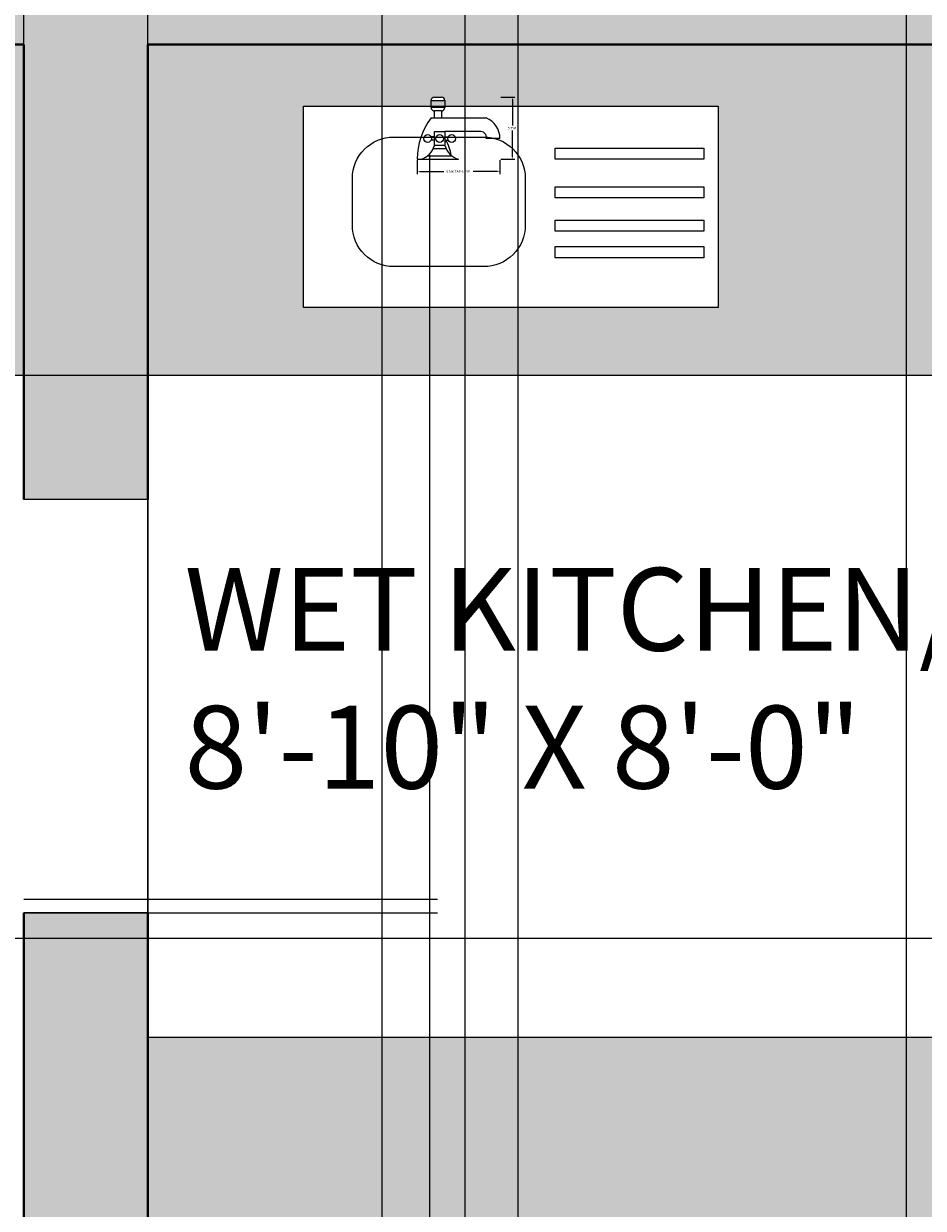
# Model space of a CAD drawing. Units: inches. Extents: x 818 to 1898, y 976 to 2364.
# Tile 89 of 96: x 1591 to 1656, y 1960 to 2046. Entities that reach past the tile are written whole.
import ezdxf

# ---------------------------------------------------------------- set-up
doc = ezdxf.new("R2010")
doc.units = ezdxf.units.IN
doc.header["$LTSCALE"] = 5
doc.header["$MEASUREMENT"] = 0
for name, color, linetype, lineweight in [('A-ANNO-DIMS', 2, 'Continuous', 18), ('A-AREA-IDEN', 7, 'Continuous', 18), ('A-DOOR', 3, 'Continuous', 25), ('A-FLOR-CASE', 8, 'Continuous', 18), ('A-FLOR-FIXT', 9, 'Continuous', 18), ('A-FURN-PATT', 8, 'Continuous', 9), ('A-WALL', 7, 'Continuous', 40)]:
    doc.layers.add(name, color=color, linetype=linetype, lineweight=lineweight)
doc.layers.add('A-WALL-PATT', color=251, linetype='Continuous', lineweight=13, true_color=0x636466)
doc.styles.get("Standard").update_dxf_attribs({"font": 'arial.ttf'})
doc.dimstyles.get("Standard").update_dxf_attribs({"dimtxt": 0.18, "dimasz": 0.18, "dimexe": 0.18, "dimexo": 0.0625, "dimgap": 0.09, "dimtad": 0, "dimtih": 1, "dimtoh": 1, "dimdec": 4, "dimzin": 0, "dimdsep": 46, "dimtxsty": 'Standard', "dimcen": 0.09, "dimadec": 0, "dimazin": 0, "dimtfac": 1, "dimtdec": 4, "dimtofl": 0, "dimtmove": 0, "dimatfit": 3, "dimfxl": 1, "dimtolj": 1, "dimtzin": 0, "dimarcsym": 0})

# ---------------------------------------------------------------- blocks, each defined once
blk = doc.blocks.new('Faucet - Bathroom side')
for p, q in [((-0.625, 4.25), (0.375, 4.25)), ((0.375, 3.75), (-0.625, 3.75)), ((-0.375, 3), (-0.375, 3.5)), ((0.125, 3.5), (0.125, 3)), ((-0.625, 3), (3.375, 3)), ((2.875, 2), (0.375, 2)), ((-0.375, 1.625), (-0.625, 1.625)), ((-0.375, 1.375), (-0.625, 1.375)), ((0.375, 1.625), (0.625, 1.625)), ((0.375, 1.375), (0.625, 1.375)), ((4.375, 1.5), (3.375, 1.5)), ((-1.625, 0), (-1.375, 0)), ((-1.375, 0), (1.375, 0)), ((-0.88366, 0.25), (0.88424, 0.25)), ((0.48078, 0.75), (-0.47286, 0.75))]:
    blk.add_line(p, q)
for points in [[(-0.375, 4.5), (0.125, 4.5)], [(-0.625, 3.75), (-0.625, 4.25)], [(0.125, 3.5), (-0.375, 3.5)], [(0.375, 4.25), (0.375, 3.75)]]:
    blk.add_lwpolyline(points)
blk.add_lwpolyline([(-0.375, 1), (-0.375, 2), (0.375, 2), (0.375, 1)], close=True)
for centre in [(-0.875, 1.5), (0, 1.5), (0.875, 1.5)]:
    blk.add_circle(centre, 0.27951)
for centre, radius, start, end in [((-0.38253, 4.2575), 0.24259, 88.22243, 181.7776), ((0.13252, 4.2575), 0.24259, 358.2224, 91.77757), ((-0.38253, 3.7424), 0.24259, 178.2224, 271.7776), ((0.13252, 3.7424), 0.24259, 268.2224, 1.777565), ((3.45929, -0.0281), 5.08436, 143.4467, 179.6834), ((2.70708, 1.4714), 1.66816, 0.9827695, 66.39737), ((2.96867, 1.5936), 0.41699, 347.0192, 102.9808), ((-1.75, 1.375), 1.42522, 285.2551, 344.7449), ((1.75, 1.375), 1.42522, 195.2551, 254.7449), ((-2.49562, -0.286), 3.38273, 9.709485, 29.48735)]:
    blk.add_arc(centre, radius, start, end)
blk = doc.blocks.new('*D38')
at = {"layer": 'A-ANNO-DIMS', "color": 0, "lineweight": -2, "ltscale": 5, "transparency": 16777216}
for p, q in [((1619.259, 2035.688), (1619.259, 2034.671)), ((1625.259, 2035.688), (1625.259, 2034.671)), ((1619.439, 2034.851), (1621.193, 2034.851)), ((1625.079, 2034.851), (1623.324, 2034.851))]:
    blk.add_line(p, q, dxfattribs=at)
at = {"layer": 'A-ANNO-DIMS', "color": 0, "ltscale": 5, "transparency": 16777216}
for points in [[(1619.439, 2034.881), (1619.439, 2034.821), (1619.259, 2034.851)], [(1625.079, 2034.881), (1625.079, 2034.821), (1625.259, 2034.851)]]:
    blk.add_solid(points, dxfattribs=at)
at = {"layer": 'Defpoints', "color": 0, "ltscale": 5, "transparency": 16777216}
for p in [(1619.259, 2035.751), (1625.259, 2035.751), (1625.259, 2034.851)]:
    blk.add_point(p, dxfattribs=at)
at = {"layer": 'A-ANNO-DIMS', "color": 0, "ltscale": 5, "transparency": 16777216, "insert": (1622.259, 2034.851), "char_height": 0.18, "attachment_point": 5}
blk.add_mtext('\\A1;SINK TAP 6 TYP.', dxfattribs=at)
blk = doc.blocks.new('*D39')
at = {"layer": 'A-ANNO-DIMS', "color": 0, "lineweight": -2, "ltscale": 5, "transparency": 16777216}
for p, q in [((1625.321, 2040.253), (1626.339, 2040.253)), ((1626.159, 2040.073), (1626.159, 2038.184)), ((1626.159, 2035.931), (1626.159, 2037.82)), ((1625.321, 2035.751), (1626.339, 2035.751))]:
    blk.add_line(p, q, dxfattribs=at)
at = {"layer": 'A-ANNO-DIMS', "color": 0, "ltscale": 5, "transparency": 16777216}
for points in [[(1626.129, 2040.073), (1626.189, 2040.073), (1626.159, 2040.253)], [(1626.129, 2035.931), (1626.189, 2035.931), (1626.159, 2035.751)]]:
    blk.add_solid(points, dxfattribs=at)
at = {"layer": 'Defpoints', "color": 0, "ltscale": 5, "transparency": 16777216}
for p in [(1625.259, 2040.253), (1626.159, 2040.253), (1625.259, 2035.751)]:
    blk.add_point(p, dxfattribs=at)
at = {"layer": 'A-ANNO-DIMS', "color": 0, "ltscale": 5, "transparency": 16777216, "insert": (1626.159, 2038.002), "char_height": 0.18, "attachment_point": 5}
blk.add_mtext('\\A1;5 TYP.', dxfattribs=at)
blk = doc.blocks.new('*D85')
at = {"layer": 'A-ANNO-DIMS', "color": 0, "lineweight": -2, "ltscale": 5, "transparency": 16777216}
for p, q in [((1258.788, 2053.078), (1897.916, 2053.078)), ((1897.736, 2052.898), (1897.736, 1876.76)), ((1897.736, 1700.258), (1897.736, 1876.396)), ((1258.788, 1700.078), (1897.916, 1700.078))]:
    blk.add_line(p, q, dxfattribs=at)
at = {"layer": 'A-ANNO-DIMS', "color": 0, "ltscale": 5, "transparency": 16777216}
for points in [[(1897.706, 2052.898), (1897.766, 2052.898), (1897.736, 2053.078)], [(1897.706, 1700.258), (1897.766, 1700.258), (1897.736, 1700.078)]]:
    blk.add_solid(points, dxfattribs=at)
at = {"layer": 'Defpoints', "color": 0, "ltscale": 5, "transparency": 16777216}
for p in [(1258.725, 2053.078), (1897.736, 2053.078), (1258.725, 1700.078)]:
    blk.add_point(p, dxfattribs=at)
at = {"layer": 'A-ANNO-DIMS', "color": 0, "ltscale": 5, "transparency": 16777216, "insert": (1897.736, 1876.578), "char_height": 0.18, "attachment_point": 5}
blk.add_mtext('\\A1;353', dxfattribs=at)
blk = doc.blocks.new('*D102')
at = {"layer": 'A-ANNO-DIMS', "color": 0, "lineweight": -2, "ltscale": 5, "transparency": 16777216}
for p, q in [((1565.483, 1071.118), (1565.483, 2363.873)), ((1626.575, 1071.118), (1626.575, 2363.873)), ((1565.663, 2363.693), (1595.635, 2363.693)), ((1626.395, 2363.693), (1596.423, 2363.693))]:
    blk.add_line(p, q, dxfattribs=at)
at = {"layer": 'A-ANNO-DIMS', "color": 0, "ltscale": 5, "transparency": 16777216}
for points in [[(1565.663, 2363.723), (1565.663, 2363.663), (1565.483, 2363.693)], [(1626.395, 2363.723), (1626.395, 2363.663), (1626.575, 2363.693)]]:
    blk.add_solid(points, dxfattribs=at)
at = {"layer": 'Defpoints', "color": 0, "ltscale": 5, "transparency": 16777216}
for p in [(1626.575, 2363.693), (1565.483, 1071.055), (1626.575, 1071.055)]:
    blk.add_point(p, dxfattribs=at)
at = {"layer": 'A-ANNO-DIMS', "color": 0, "ltscale": 5, "transparency": 16777216, "insert": (1596.029, 2363.693), "char_height": 0.18, "attachment_point": 5}
blk.add_mtext('\\A1;61.09', dxfattribs=at)
blk = doc.blocks.new('*D103')
at = {"layer": 'A-ANNO-DIMS', "color": 0, "lineweight": -2, "ltscale": 5, "transparency": 16777216}
for p, q in [((1626.575, 1071.118), (1626.575, 2363.873)), ((1689.471, 1071.118), (1689.471, 2363.873)), ((1626.755, 2363.693), (1657.699, 2363.693)), ((1689.291, 2363.693), (1658.348, 2363.693))]:
    blk.add_line(p, q, dxfattribs=at)
at = {"layer": 'A-ANNO-DIMS', "color": 0, "ltscale": 5, "transparency": 16777216}
for points in [[(1626.755, 2363.723), (1626.755, 2363.663), (1626.575, 2363.693)], [(1689.291, 2363.723), (1689.291, 2363.663), (1689.471, 2363.693)]]:
    blk.add_solid(points, dxfattribs=at)
at = {"layer": 'Defpoints', "color": 0, "ltscale": 5, "transparency": 16777216}
for p in [(1689.471, 2363.693), (1626.575, 1071.055), (1689.471, 1071.055)]:
    blk.add_point(p, dxfattribs=at)
at = {"layer": 'A-ANNO-DIMS', "color": 0, "ltscale": 5, "transparency": 16777216, "insert": (1658.023, 2363.693), "char_height": 0.18, "attachment_point": 5}
blk.add_mtext('\\A1;62.9', dxfattribs=at)
blk = doc.blocks.new('*D173')
at = {"layer": 'A-ANNO-DIMS', "color": 0, "lineweight": -2, "ltscale": 5, "transparency": 16777216}
for p, q in [((1622.725, 1463.141), (1622.725, 2363.873)), ((1654.725, 1463.141), (1654.725, 2363.873)), ((1622.905, 2363.693), (1638.507, 2363.693)), ((1654.545, 2363.693), (1638.943, 2363.693))]:
    blk.add_line(p, q, dxfattribs=at)
at = {"layer": 'A-ANNO-DIMS', "color": 0, "ltscale": 5, "transparency": 16777216}
for points in [[(1622.905, 2363.723), (1622.905, 2363.663), (1622.725, 2363.693)], [(1654.545, 2363.723), (1654.545, 2363.663), (1654.725, 2363.693)]]:
    blk.add_solid(points, dxfattribs=at)
at = {"layer": 'Defpoints', "color": 0, "ltscale": 5, "transparency": 16777216}
for p in [(1654.725, 2363.693), (1622.725, 1463.078), (1654.725, 1463.078)]:
    blk.add_point(p, dxfattribs=at)
at = {"layer": 'A-ANNO-DIMS', "color": 0, "ltscale": 5, "transparency": 16777216, "insert": (1638.725, 2363.693), "char_height": 0.18, "attachment_point": 5}
blk.add_mtext('\\A1;32', dxfattribs=at)
blk = doc.blocks.new('*D174')
at = {"layer": 'A-ANNO-DIMS', "color": 0, "lineweight": -2, "ltscale": 5, "transparency": 16777216}
for p, q in [((1616.725, 1416.748), (1616.725, 2363.873)), ((1622.725, 1416.748), (1622.725, 2363.873)), ((1616.905, 2363.693), (1619.576, 2363.693)), ((1622.545, 2363.693), (1619.875, 2363.693))]:
    blk.add_line(p, q, dxfattribs=at)
at = {"layer": 'A-ANNO-DIMS', "color": 0, "ltscale": 5, "transparency": 16777216}
for points in [[(1616.905, 2363.723), (1616.905, 2363.663), (1616.725, 2363.693)], [(1622.545, 2363.723), (1622.545, 2363.663), (1622.725, 2363.693)]]:
    blk.add_solid(points, dxfattribs=at)
at = {"layer": 'Defpoints', "color": 0, "ltscale": 5, "transparency": 16777216}
for p in [(1622.725, 2363.693), (1616.725, 1416.686), (1622.725, 1416.686)]:
    blk.add_point(p, dxfattribs=at)
at = {"layer": 'A-ANNO-DIMS', "color": 0, "ltscale": 5, "transparency": 16777216, "insert": (1619.725, 2363.693), "char_height": 0.18, "attachment_point": 5}
blk.add_mtext('\\A1;6', dxfattribs=at)
blk = doc.blocks.new('*D175')
at = {"layer": 'A-ANNO-DIMS', "color": 0, "lineweight": -2, "ltscale": 5, "transparency": 16777216}
for p, q in [((1559.725, 1647.641), (1559.725, 2363.873)), ((1669.725, 1647.641), (1669.725, 2363.873)), ((1559.905, 2363.693), (1614.445, 2363.693)), ((1669.545, 2363.693), (1615.005, 2363.693))]:
    blk.add_line(p, q, dxfattribs=at)
at = {"layer": 'A-ANNO-DIMS', "color": 0, "ltscale": 5, "transparency": 16777216}
for points in [[(1559.905, 2363.723), (1559.905, 2363.663), (1559.725, 2363.693)], [(1669.545, 2363.723), (1669.545, 2363.663), (1669.725, 2363.693)]]:
    blk.add_solid(points, dxfattribs=at)
at = {"layer": 'Defpoints', "color": 0, "ltscale": 5, "transparency": 16777216}
for p in [(1669.725, 2363.693), (1559.725, 1647.578), (1669.725, 1647.578)]:
    blk.add_point(p, dxfattribs=at)
at = {"layer": 'A-ANNO-DIMS', "color": 0, "ltscale": 5, "transparency": 16777216, "insert": (1614.725, 2363.693), "char_height": 0.18, "attachment_point": 5}
blk.add_mtext('\\A1;110', dxfattribs=at)
blk = doc.blocks.new('*D203')
at = {"layer": 'A-ANNO-DIMS', "color": 0, "lineweight": -2, "ltscale": 5, "transparency": 16777216}
for p, q in [((1599.725, 1876.141), (1599.725, 2363.873)), ((1705.725, 1876.141), (1705.725, 2363.873)), ((1599.905, 2363.693), (1652.445, 2363.693)), ((1705.545, 2363.693), (1653.005, 2363.693))]:
    blk.add_line(p, q, dxfattribs=at)
at = {"layer": 'A-ANNO-DIMS', "color": 0, "ltscale": 5, "transparency": 16777216}
for points in [[(1599.905, 2363.723), (1599.905, 2363.663), (1599.725, 2363.693)], [(1705.545, 2363.723), (1705.545, 2363.663), (1705.725, 2363.693)]]:
    blk.add_solid(points, dxfattribs=at)
at = {"layer": 'Defpoints', "color": 0, "ltscale": 5, "transparency": 16777216}
for p in [(1705.725, 2363.693), (1599.725, 1876.078), (1705.725, 1876.078)]:
    blk.add_point(p, dxfattribs=at)
at = {"layer": 'A-ANNO-DIMS', "color": 0, "ltscale": 5, "transparency": 16777216, "insert": (1652.725, 2363.693), "char_height": 0.18, "attachment_point": 5}
blk.add_mtext('\\A1;106', dxfattribs=at)
blk = doc.blocks.new('*D205')
at = {"layer": 'A-ANNO-DIMS', "color": 0, "lineweight": -2, "ltscale": 5, "transparency": 16777216}
for p, q in [((1590.725, 2044.141), (1590.725, 2363.873)), ((1714.725, 2053.141), (1714.725, 2363.873)), ((1590.905, 2363.693), (1652.445, 2363.693)), ((1714.545, 2363.693), (1653.005, 2363.693))]:
    blk.add_line(p, q, dxfattribs=at)
at = {"layer": 'A-ANNO-DIMS', "color": 0, "ltscale": 5, "transparency": 16777216}
for points in [[(1590.905, 2363.723), (1590.905, 2363.663), (1590.725, 2363.693)], [(1714.545, 2363.723), (1714.545, 2363.663), (1714.725, 2363.693)]]:
    blk.add_solid(points, dxfattribs=at)
at = {"layer": 'Defpoints', "color": 0, "ltscale": 5, "transparency": 16777216}
for p in [(1714.725, 2363.693), (1714.725, 2053.078), (1590.725, 2044.078)]:
    blk.add_point(p, dxfattribs=at)
at = {"layer": 'A-ANNO-DIMS', "color": 0, "ltscale": 5, "transparency": 16777216, "insert": (1652.725, 2363.693), "char_height": 0.18, "attachment_point": 5}
blk.add_mtext('\\A1;124', dxfattribs=at)
blk = doc.blocks.new('*D208')
at = {"layer": 'A-ANNO-DIMS', "color": 0, "lineweight": -2, "ltscale": 5, "transparency": 16777216}
for p, q in [((1599.788, 2044.078), (1897.916, 2044.078)), ((1897.736, 2043.898), (1897.736, 2032.259)), ((1897.736, 2020.258), (1897.736, 2031.898)), ((1599.788, 2020.078), (1897.916, 2020.078))]:
    blk.add_line(p, q, dxfattribs=at)
at = {"layer": 'A-ANNO-DIMS', "color": 0, "ltscale": 5, "transparency": 16777216}
for points in [[(1897.706, 2043.898), (1897.766, 2043.898), (1897.736, 2044.078)], [(1897.706, 2020.258), (1897.766, 2020.258), (1897.736, 2020.078)]]:
    blk.add_solid(points, dxfattribs=at)
at = {"layer": 'Defpoints', "color": 0, "ltscale": 5, "transparency": 16777216}
for p in [(1599.725, 2044.078), (1897.736, 2044.078), (1599.725, 2020.078)]:
    blk.add_point(p, dxfattribs=at)
at = {"layer": 'A-ANNO-DIMS', "color": 0, "ltscale": 5, "transparency": 16777216, "insert": (1897.736, 2032.078), "char_height": 0.18, "attachment_point": 5}
blk.add_mtext('\\A1;24', dxfattribs=at)
blk = doc.blocks.new('*D229')
at = {"layer": 'A-ANNO-DIMS', "color": 0, "lineweight": -2, "ltscale": 5, "transparency": 16777216}
for p, q in [((1599.725, 2044.016), (1599.725, 975.663)), ((1620.142, 2036.056), (1620.142, 975.663)), ((1599.905, 975.843), (1609.468, 975.843)), ((1619.962, 975.843), (1610.398, 975.843))]:
    blk.add_line(p, q, dxfattribs=at)
at = {"layer": 'A-ANNO-DIMS', "color": 0, "ltscale": 5, "transparency": 16777216}
for points in [[(1599.905, 975.873), (1599.905, 975.813), (1599.725, 975.843)], [(1619.962, 975.873), (1619.962, 975.813), (1620.142, 975.843)]]:
    blk.add_solid(points, dxfattribs=at)
at = {"layer": 'Defpoints', "color": 0, "ltscale": 5, "transparency": 16777216}
for p in [(1599.725, 2044.078), (1620.142, 2036.118), (1620.142, 975.843)]:
    blk.add_point(p, dxfattribs=at)
at = {"layer": 'A-ANNO-DIMS', "color": 0, "ltscale": 5, "transparency": 16777216, "insert": (1609.933, 975.843), "char_height": 0.18, "attachment_point": 5}
blk.add_mtext('\\A1;20.416', dxfattribs=at)
blk = doc.blocks.new('*D239')
at = {"layer": 'A-ANNO-DIMS', "color": 0, "lineweight": -2, "ltscale": 5, "transparency": 16777216}
for p, q in [((1483.608, 1979.244), (1897.916, 1979.244)), ((1897.736, 1979.064), (1897.736, 1964.134)), ((1897.736, 1948.84), (1897.736, 1963.77)), ((1483.608, 1948.66), (1897.916, 1948.66))]:
    blk.add_line(p, q, dxfattribs=at)
at = {"layer": 'A-ANNO-DIMS', "color": 0, "ltscale": 5, "transparency": 16777216}
for points in [[(1897.706, 1979.064), (1897.766, 1979.064), (1897.736, 1979.244)], [(1897.706, 1948.84), (1897.766, 1948.84), (1897.736, 1948.66)]]:
    blk.add_solid(points, dxfattribs=at)
at = {"layer": 'Defpoints', "color": 0, "ltscale": 5, "transparency": 16777216}
for p in [(1483.545, 1979.244), (1897.736, 1979.244), (1483.545, 1948.66)]:
    blk.add_point(p, dxfattribs=at)
at = {"layer": 'A-ANNO-DIMS', "color": 0, "ltscale": 5, "transparency": 16777216, "insert": (1897.736, 1963.952), "char_height": 0.18, "attachment_point": 5}
blk.add_mtext('\\A1;30.584', dxfattribs=at)
blk = doc.blocks.new('*D241')
at = {"layer": 'A-ANNO-DIMS', "color": 0, "lineweight": -2, "ltscale": 5, "transparency": 16777216}
for p, q in [((1590.788, 2020.078), (1897.916, 2020.078)), ((1897.736, 2019.898), (1897.736, 1999.843)), ((1897.736, 1979.424), (1897.736, 1999.479)), ((1550.073, 1979.244), (1897.916, 1979.244))]:
    blk.add_line(p, q, dxfattribs=at)
at = {"layer": 'A-ANNO-DIMS', "color": 0, "ltscale": 5, "transparency": 16777216}
for points in [[(1897.706, 2019.898), (1897.766, 2019.898), (1897.736, 2020.078)], [(1897.706, 1979.424), (1897.766, 1979.424), (1897.736, 1979.244)]]:
    blk.add_solid(points, dxfattribs=at)
at = {"layer": 'Defpoints', "color": 0, "ltscale": 5, "transparency": 16777216}
for p in [(1590.725, 2020.078), (1897.736, 2020.078), (1550.011, 1979.244)]:
    blk.add_point(p, dxfattribs=at)
at = {"layer": 'A-ANNO-DIMS', "color": 0, "ltscale": 5, "transparency": 16777216, "insert": (1897.736, 1999.661), "char_height": 0.18, "attachment_point": 5}
blk.add_mtext('\\A1;40.83', dxfattribs=at)
blk = doc.blocks.new('*D282')
at = {"layer": 'A-ANNO-DIMS', "color": 0, "lineweight": -2, "ltscale": 5, "transparency": 16777216}
for p, q in [((1422.083, 2081.188), (1897.916, 2081.188)), ((1897.736, 2081.008), (1897.736, 1884.315)), ((1897.736, 1687.258), (1897.736, 1883.951)), ((1463.788, 1687.078), (1897.916, 1687.078))]:
    blk.add_line(p, q, dxfattribs=at)
at = {"layer": 'A-ANNO-DIMS', "color": 0, "ltscale": 5, "transparency": 16777216}
for points in [[(1897.706, 2081.008), (1897.766, 2081.008), (1897.736, 2081.188)], [(1897.706, 1687.258), (1897.766, 1687.258), (1897.736, 1687.078)]]:
    blk.add_solid(points, dxfattribs=at)
at = {"layer": 'Defpoints', "color": 0, "ltscale": 5, "transparency": 16777216}
for p in [(1422.02, 2081.188), (1897.736, 2081.188), (1463.725, 1687.078)]:
    blk.add_point(p, dxfattribs=at)
at = {"layer": 'A-ANNO-DIMS', "color": 0, "ltscale": 5, "transparency": 16777216, "insert": (1897.736, 1884.133), "char_height": 0.18, "attachment_point": 5}
blk.add_mtext('\\A1;394.1', dxfattribs=at)

msp = doc.modelspace()

# ---------------------------------------------------------------- hatches: boundary and pattern name
at = {"layer": 'A-FURN-PATT', "ltscale": 5}
h = msp.add_hatch(color=256, dxfattribs=at)
h.dxf.hatch_style = 1
h.paths.add_polyline_path([(1341.9997, 1981.5338), (1317.9034, 2001.8247), (1314.2595, 2001.8247), (1314.2595, 2004.893), (1310.1046, 2008.3917), (1303.9314, 2008.3917), (1303.9314, 1953.0408), (1308.1629, 1953.0408), (1314.2595, 1958.1746), (1314.2595, 1959.6079), (1315.9616, 1959.6079)])
h.paths.add_polyline_path([(1341.9997, 1981.5338), (1315.9616, 1959.6079), (1336.7936, 1959.6079), (1336.7936, 1953.0408), (1345.3966, 1953.0408), (1345.3966, 1959.6079), (1368.0379, 1959.6079)])
h.paths.add_polyline_path([(1402.518, 2008.3917), (1398.8475, 2008.3917), (1398.8475, 2001.8247), (1376.3134, 2001.8247), (1376.3134, 2008.3917), (1373.8948, 2008.3917), (1367.9307, 2003.3695), (1367.9307, 2001.8247), (1366.0961, 2001.8247), (1341.9997, 1981.5338), (1368.0379, 1959.6079), (1375.8366, 1953.0408), (1376.3134, 1953.0408), (1376.3134, 1959.6079), (1398.8475, 1959.6079), (1398.8475, 1953.0408), (1402.518, 1953.0408)])
h.paths.add_polyline_path([(1366.0961, 2001.8247), (1345.3966, 2001.8247), (1345.3966, 2008.3917), (1336.7936, 2008.3917), (1336.7936, 2001.8247), (1317.9034, 2001.8247), (1341.9997, 1981.5338)])
h.paths.add_polyline_path([(1336.7936, 1959.6079), (1315.9616, 1959.6079), (1314.2595, 1958.1746), (1314.2595, 1953.0408), (1336.7936, 1953.0408)], flags=17)
h.paths.add_polyline_path([(1367.9307, 1959.6079), (1345.3966, 1959.6079), (1345.3966, 1953.0408), (1367.9307, 1953.0408)], flags=17)
h.paths.add_polyline_path([(1398.8475, 1959.6079), (1376.3134, 1959.6079), (1376.3134, 1953.0408), (1398.8475, 1953.0408)], flags=17)
h.paths.add_polyline_path([(1368.0379, 1959.6079), (1367.9307, 1959.6079), (1367.9307, 1953.0408), (1375.8366, 1953.0408)], flags=17)
h.paths.add_polyline_path([(1314.2595, 1958.1746), (1308.1629, 1953.0408), (1314.2595, 1953.0408)], flags=17)
h.paths.add_polyline_path([(1315.9616, 1959.6079), (1314.2595, 1959.6079), (1314.2595, 1958.1746)], flags=16)
h.paths.add_polyline_path([(1314.2595, 2008.3917), (1310.1046, 2008.3917), (1314.2595, 2004.893)], flags=17)
h.paths.add_polyline_path([(1336.7936, 2008.3917), (1314.2595, 2008.3917), (1314.2595, 2004.893), (1317.9034, 2001.8247), (1336.7936, 2001.8247)], flags=17)
h.paths.add_polyline_path([(1314.2595, 2004.893), (1314.2595, 2001.8247), (1317.9034, 2001.8247)], flags=16)
h.paths.add_polyline_path([(1367.9307, 2008.3917), (1345.3966, 2008.3917), (1345.3966, 2001.8247), (1366.0961, 2001.8247), (1367.9307, 2003.3695)], flags=17)
h.paths.add_polyline_path([(1398.8475, 2008.3917), (1376.3134, 2008.3917), (1376.3134, 2001.8247), (1398.8475, 2001.8247)], flags=17)
h.paths.add_polyline_path([(1373.8948, 2008.3917), (1367.9307, 2008.3917), (1367.9307, 2003.3695)], flags=17)
h.paths.add_polyline_path([(1367.9307, 2003.3695), (1366.0961, 2001.8247), (1367.9307, 2001.8247)], flags=16)
h.paths.add_polyline_path([(1546.1595, 2044.0782), (1451.7698, 2044.0782), (1451.7698, 2020.0782), (1546.1595, 2020.0782)])
h.paths.add_polyline_path([(1492.0729, 2040.001, 0.431429), (1491.8238, 2040.251), (1491.3087, 2040.251, 0.415217), (1491.0729, 2040.001)], flags=16)
h.paths.add_polyline_path([(1481.8346, 2039.6036), (1511.886, 2039.6036), (1511.886, 2024.9917), (1481.8346, 2024.9917)], flags=16)
h.paths.add_polyline_path([(1491.0729, 2039.4857), (1491.0729, 2039.501), (1492.0729, 2039.501, -0.4117484), (1491.8401, 2039.251), (1491.8229, 2039.251), (1491.8229, 2039.2509, 0.4325918), (1492.0729, 2039.501), (1491.0729, 2039.501, 0.432604), (1491.3229, 2039.2509), (1491.3229, 2039.251), (1491.325, 2039.251, -0.4165823)], flags=0)
h.paths.add_polyline_path([(1485.3701, 2030.9622), (1485.3701, 2034.3556, -0.4142136), (1488.3701, 2037.3556), (1490.3421, 2037.3556, -0.0779193), (1491.0729, 2038.751), (1495.0729, 2038.751, -0.3148679), (1496.07, 2037.1201, -0.3016609), (1497.9049, 2034.3556), (1497.9049, 2030.9622, -0.4142136), (1494.9049, 2027.9622), (1488.3701, 2027.9622, -0.4142136)], flags=0)
h.paths.add_polyline_path([(1490.3229, 2035.751, 0.2655648), (1491.3229, 2036.751), (1491.3229, 2037.126), (1491.0729, 2037.126, -0.7914183), (1490.5434, 2037.251, -0.7914183), (1491.0729, 2037.376), (1491.3229, 2037.376), (1491.3229, 2037.751), (1492.0729, 2037.751), (1492.0729, 2037.376), (1492.3229, 2037.376, -0.7914183), (1492.8524, 2037.251, -0.7914183), (1492.3229, 2037.126), (1492.1491, 2037.126, -0.0866263), (1492.5376, 2036.0294, 0.1070481), (1493.0729, 2035.751), (1490.3229, 2035.751)], flags=0)
h.paths.add_polyline_path([(1491.9774, 2037.251, -1), (1491.4184, 2037.251, -1)], flags=0)
h.paths.add_polyline_path([(1500.0743, 2028.6045), (1500.0743, 2029.4074), (1510.8414, 2029.4074), (1510.8414, 2028.6045)], flags=0)
h.paths.add_polyline_path([(1500.0743, 2030.5314), (1500.0743, 2031.3342), (1510.8414, 2031.3342), (1510.8414, 2030.5314)], flags=0)
h.paths.add_polyline_path([(1500.0743, 2032.94), (1500.0743, 2033.7428), (1510.8414, 2033.7428), (1510.8414, 2032.94)], flags=0)
h.paths.add_polyline_path([(1500.0743, 2035.7499), (1500.0743, 2036.5528), (1510.8414, 2036.5528), (1510.8414, 2035.7499)], flags=0)
h.paths.add_polyline_path([(1590.7251, 2044.0782), (1576.1595, 2044.0782), (1576.1595, 2020.0782), (1590.7251, 2020.0782)])
h.paths.add_polyline_path([(1668.4429, 2044.0782), (1599.7251, 2044.0782), (1599.7251, 2020.0782), (1668.4429, 2020.0782)])
h.paths.add_polyline_path([(1621.2588, 2040.001, 0.431429), (1621.0097, 2040.251), (1620.4946, 2040.251, 0.415217), (1620.2588, 2040.001)], flags=16)
h.paths.add_polyline_path([(1611.0205, 2024.9917), (1611.0205, 2039.6036), (1641.0719, 2039.6036), (1641.0719, 2024.9917)], flags=16)
h.paths.add_polyline_path([(1620.2588, 2039.4857), (1620.2588, 2039.501), (1621.2588, 2039.501, -0.4117484), (1621.026, 2039.251), (1621.0088, 2039.251), (1621.0088, 2039.2509, 0.4325918), (1621.2588, 2039.501), (1620.2588, 2039.501, 0.432604), (1620.5088, 2039.2509), (1620.5088, 2039.251), (1620.5109, 2039.251, -0.4165823)], flags=0)
h.paths.add_polyline_path([(1614.556, 2030.9622), (1614.556, 2034.3556, -0.4142136), (1617.556, 2037.3556), (1619.528, 2037.3556, -0.0779193), (1620.2588, 2038.751), (1624.2588, 2038.751, -0.3148679), (1625.2559, 2037.1201, -0.3016609), (1627.0908, 2034.3556), (1627.0908, 2030.9622, -0.4142136), (1624.0908, 2027.9622), (1617.556, 2027.9622, -0.4142136)], flags=0)
h.paths.add_polyline_path([(1619.5088, 2035.751, 0.2655648), (1620.5088, 2036.751), (1620.5088, 2037.126), (1620.2588, 2037.126, -0.7914183), (1619.7293, 2037.251, -0.7914183), (1620.2588, 2037.376), (1620.5088, 2037.376), (1620.5088, 2037.751), (1621.2588, 2037.751), (1621.2588, 2037.376), (1621.5088, 2037.376, -0.7914183), (1622.0383, 2037.251, -0.7914183), (1621.5088, 2037.126), (1621.335, 2037.126, -0.0866263), (1621.7235, 2036.0294, 0.1070481), (1622.2588, 2035.751), (1619.5088, 2035.751)], flags=0)
h.paths.add_polyline_path([(1620.6043, 2037.251, -1), (1621.1633, 2037.251, -1)], flags=0)
h.paths.add_polyline_path([(1629.2602, 2028.6045), (1629.2602, 2029.4074), (1640.0273, 2029.4074), (1640.0273, 2028.6045)], flags=0)
h.paths.add_polyline_path([(1629.2602, 2030.5314), (1629.2602, 2031.3342), (1640.0273, 2031.3342), (1640.0273, 2030.5314)], flags=0)
h.paths.add_polyline_path([(1629.2602, 2032.94), (1629.2602, 2033.7428), (1640.0273, 2033.7428), (1640.0273, 2032.94)], flags=0)
h.paths.add_polyline_path([(1629.2602, 2035.7499), (1629.2602, 2036.5528), (1640.0273, 2036.5528), (1640.0273, 2035.7499)], flags=0)
h.paths.add_polyline_path([(1705.7251, 2044.0782), (1698.4429, 2044.0782), (1698.4429, 2020.0782), (1705.7251, 2020.0782)])
h.paths.add_polyline_path([(1705.7251, 1972.0782), (1599.7251, 1972.0782), (1599.7251, 1948.0782), (1705.7251, 1948.0782)])
h.paths.add_polyline_path([(1550.0109, 1979.2444), (1483.5451, 1979.2444), (1483.5451, 1948.6602), (1550.0109, 1948.6602)])
h.paths.add_polyline_path([(1490.2586, 1948.6602), (1488.2586, 1948.6602), (1488.2586, 1941.1742, 0.4142136), (1491.2586, 1938.1742), (1500.7446, 1938.1742, -0.4142136)])
h.paths.add_polyline_path([(1513.2306, 1941.1742), (1513.2306, 1948.6602), (1511.2306, 1948.6602, -0.4142136), (1500.7446, 1938.1742), (1510.2306, 1938.1742, 0.4142136)])
h.paths.add_polyline_path([(1518.778, 1948.6602), (1516.778, 1948.6602), (1516.778, 1941.1742, 0.4142136), (1519.778, 1938.1742), (1529.264, 1938.1742, -0.4142136)])
h.paths.add_polyline_path([(1541.75, 1941.1742), (1541.75, 1948.6602), (1539.75, 1948.6602, -0.4142136), (1529.264, 1938.1742), (1538.75, 1938.1742, 0.4142136)])
h.paths.add_polyline_path([(1590.7251, 1900.0782), (1519.6413, 1900.0782), (1519.6413, 1876.0782), (1590.7251, 1876.0782)])
at = {"layer": 'A-WALL-PATT', "ltscale": 5}
h = msp.add_hatch(color=256, dxfattribs=at)
h.dxf.hatch_style = 1
h.paths.add_polyline_path([(1267.7252, 1928.9218), (1258.7251, 1928.9218), (1258.7251, 1913.6401), (1250.3029, 1913.6401), (1250.3029, 1878.3919), (1258.7251, 1878.3919), (1258.7251, 1862.9652), (1267.7252, 1862.9652)])
h.paths.add_polyline_path([(1267.7252, 1814.9652), (1258.7251, 1814.9652), (1258.7251, 1755.3321), (1267.7252, 1755.3321)])
h.paths.add_polyline_path([(1463.7251, 1696.0782), (1267.7252, 1696.0782), (1267.7252, 1707.3321), (1258.7251, 1707.3321), (1258.7251, 1700.0782), (1251.9333, 1700.0782), (1251.9333, 1687.0782), (1463.7251, 1687.0782)])
h.paths.add_polyline_path([(1714.7251, 1717.3178), (1705.7251, 1717.3178), (1705.7251, 1696.0782), (1599.7251, 1696.0782), (1599.7251, 1790.0782), (1705.7251, 1790.0782), (1705.7251, 1785.6125), (1714.7251, 1785.6125), (1714.7251, 1827.2125), (1705.7251, 1827.2125), (1705.7251, 1802.0782), (1599.7251, 1802.0782), (1599.7251, 1867.0782), (1705.7251, 1867.0782), (1705.7251, 1857.2125), (1714.7251, 1857.2125), (1714.7251, 1930.0316), (1741.8409, 1930.0316), (1741.8409, 1935.0316), (1714.7251, 1935.0316), (1714.7251, 1957.0338), (1741.8409, 1957.0338), (1741.8409, 1962.0338), (1714.7251, 1962.0338), (1705.7251, 1962.0338), (1705.7251, 1948.0782), (1599.7251, 1948.0782), (1599.7251, 1981.0782), (1590.7251, 1981.0782), (1590.7251, 1941.0782), (1620.7252, 1941.0782), (1705.7251, 1941.0782), (1705.7251, 1876.0782), (1599.7251, 1876.0782), (1599.7251, 1911.0782), (1590.7251, 1911.0782), (1590.7251, 1876.0782), (1429.2252, 1876.0782), (1429.2252, 1867.0782), (1511.7252, 1867.0782), (1528.593, 1867.0782), (1595.7252, 1867.0782), (1595.7252, 1773.0782), (1520.7252, 1773.0782), (1520.7252, 1837.5823), (1532.593, 1837.5823), (1532.593, 1867.0782), (1528.593, 1867.0782), (1528.593, 1841.5823), (1511.7252, 1841.5823), (1511.7252, 1744.9714), (1520.7252, 1744.9714), (1520.7252, 1761.0782), (1595.7252, 1761.0782), (1595.7252, 1696.0782), (1520.7252, 1696.0782), (1520.7252, 1716.0454), (1511.7252, 1716.0454), (1511.7252, 1696.0782), (1511.7252, 1687.0782), (1714.7251, 1687.0782)])
h.paths.add_polyline_path([(1714.7251, 2053.0782), (1714.7251, 2081.1881), (1709.7252, 2081.1881), (1709.7252, 2053.0782), (1681.6446, 2053.0782), (1681.6446, 2081.1881), (1676.6446, 2081.1881), (1676.6446, 2053.0782), (1538.5155, 2053.0782), (1538.5155, 2044.0782), (1590.7251, 2044.0782), (1590.7251, 2011.0782), (1599.7251, 2011.0782), (1599.7251, 2044.0782), (1705.7251, 2044.0782), (1705.7251, 2014.5114), (1714.7251, 2014.5114)])
h.paths.add_polyline_path([(1485.1216, 2053.0782), (1422.02, 2053.0782), (1422.02, 2081.1881), (1413.02, 2081.1881), (1413.02, 2053.0782), (1399.6356, 2053.0782), (1399.6356, 2081.1881), (1390.6356, 2081.1881), (1390.6356, 2053.0782), (1388.0315, 2053.0782), (1388.0315, 2044.0782), (1416.2743, 2044.0782), (1485.1216, 2044.0782)])
h.paths.add_polyline_path([(1330.305, 2053.0782), (1258.7251, 2053.0782), (1258.7251, 2019.2871), (1267.7252, 2019.2871), (1267.7252, 2044.0782), (1330.305, 2044.0782)])
h.paths.add_polyline_path([(1258.7251, 2053.0782), (1214.6577, 2053.0782), (1214.6577, 2044.0782), (1258.7251, 2044.0782)])
h.paths.add_polyline_path([(1214.6577, 2053.0782), (1180.349, 2053.0782), (1180.349, 2044.0782), (1214.6577, 2044.0782)])
h.paths.add_polyline_path([(1714.7251, 1639.5782), (1741.8409, 1639.5782), (1741.8409, 1643.5782), (1714.7251, 1643.5782), (1714.7251, 1649.9029), (1705.7251, 1649.9029), (1705.7251, 1600.0782), (1477.7252, 1600.0782), (1477.7252, 1591.0782), (1520.7252, 1591.0782), (1616.7251, 1591.0782), (1616.7251, 1416.6857), (1622.7251, 1416.6857), (1622.7251, 1463.0782), (1624.7252, 1463.0782), (1624.7252, 1467.0782), (1622.7251, 1467.0782), (1622.7251, 1591.0782), (1705.7251, 1591.0782), (1705.7251, 1545.0782), (1714.7251, 1545.0782), (1741.8409, 1545.0782), (1741.8409, 1549.0782), (1714.7251, 1549.0782), (1714.7251, 1593.9175), (1737.8409, 1593.9175), (1737.8409, 1597.9175), (1714.7251, 1597.9175)])
h.paths.add_polyline_path([(1674.9024, 2060.7419), (1714.7045, 2060.7419), (1714.7045, 2073.1061), (1674.9024, 2073.1061)], flags=25)
h.paths.add_polyline_path([(1394.5468, 2061.6618), (1422.2344, 2061.6618), (1422.2344, 2074.0261), (1394.5468, 2074.0261)], flags=24)

# ---------------------------------------------------------------- linework, layer by layer
at = {"layer": 'A-DOOR'}
for p, q in [((1599.7251, 2011.0782), (1590.7251, 2011.0782)), ((1590.7251, 1982.0782), (1620.7252, 1982.0782)), ((1599.7251, 1981.0782), (1590.7251, 1981.0782)), ((1590.7251, 1981.0782), (1620.7252, 1981.0782))]:
    msp.add_line(p, q, dxfattribs=at)
at = {"layer": 'A-FLOR-CASE'}
for p, q in [((1451.7698, 2020.0782), (1590.7251, 2020.0782)), ((1599.7251, 2020.0782), (1705.7251, 2020.0782)), ((1599.7251, 1972.0782), (1705.7251, 1972.0782))]:
    msp.add_line(p, q, dxfattribs=at)
at = {"layer": 'A-FLOR-FIXT'}
for points in [[(1611.0205, 2039.6036), (1641.0719, 2039.6036), (1641.0719, 2024.9917), (1611.0205, 2024.9917)], [(1629.2602, 2036.5528), (1640.0273, 2036.5528), (1640.0273, 2035.7499), (1629.2602, 2035.7499)], [(1629.2602, 2033.7428), (1640.0273, 2033.7428), (1640.0273, 2032.94), (1629.2602, 2032.94)], [(1629.2602, 2031.3342), (1640.0273, 2031.3342), (1640.0273, 2030.5314), (1629.2602, 2030.5314)], [(1629.2602, 2029.4074), (1640.0273, 2029.4074), (1640.0273, 2028.6045), (1629.2602, 2028.6045)]]:
    msp.add_lwpolyline(points, close=True, dxfattribs=at)
msp.add_lwpolyline([(1617.556, 2037.3556), (1624.0908, 2037.3556, -0.4142136), (1627.0908, 2034.3556), (1627.0908, 2030.9622, -0.4142136), (1624.0908, 2027.9622), (1617.556, 2027.9622, -0.4142136), (1614.556, 2030.9622), (1614.556, 2034.3556, -0.4142136)], format="xyb", close=True, dxfattribs=at)
at = {"layer": 'A-WALL'}
for p, q in [((1267.7252, 2044.0782), (1590.7251, 2044.0782)), ((1590.7251, 2044.0782), (1590.7251, 2011.0782)), ((1599.7251, 2044.0782), (1599.7251, 2011.0782)), ((1599.7251, 2044.0782), (1705.7251, 2044.0782)), ((1599.7251, 2044.0782), (1599.7251, 2011.0782)), ((1590.7251, 1981.0782), (1590.7251, 1941.0782)), ((1599.7251, 1981.0782), (1599.7251, 1948.0782)), ((1599.7251, 1981.0782), (1599.7251, 1948.0782))]:
    msp.add_line(p, q, dxfattribs=at)

# ---------------------------------------------------------------- block references
at = {"layer": 'A-FLOR-FIXT'}
msp.add_blockref('Faucet - Bathroom side', (1620.8838, 2035.751), dxfattribs=at)

# ---------------------------------------------------------------- texts
at = {"layer": 'A-AREA-IDEN', "ltscale": 5, "insert": (1602.387, 2006.1043), "char_height": 6, "attachment_point": 1}
msp.add_mtext_dynamic_manual_height_columns('WET KITCHEN/UTILITY\\P8\'-10" X 8\'-0"', width=118.992422, gutter_width=1, heights=[0], dxfattribs=at)

# ---------------------------------------------------------------- dimensions: what is measured, and where the dimension line sits
at = {"layer": 'A-ANNO-DIMS', "ltscale": 5}
for base, p1, p2, override, picture, middle in [((1669.7251, 2363.6929), (1559.7251, 1647.5782), (1669.7251, 1647.5782), {"dimdec": 0, "dimlfac": 1, "dimrnd": 0, "dimzin": 0, "dimdsep": 46, "dimlunit": 2}, '*D175', (1614.7251, 2363.6929)), ((1626.5748, 2363.6929), (1565.4835, 1071.0552), (1626.5748, 1071.0552), {"dimdec": 2, "dimlfac": 1, "dimrnd": 0, "dimzin": 0, "dimdsep": 46, "dimlunit": 2}, '*D102', (1596.0291, 2363.6929)), ((1714.7251, 2363.6929), (1590.7251, 2044.0782), (1714.7251, 2053.0782), {"dimdec": 0, "dimlfac": 1, "dimrnd": 0, "dimzin": 0, "dimdsep": 46, "dimlunit": 2}, '*D205', (1652.7251, 2363.6929)), ((1705.7251, 2363.6929), (1599.7251, 1876.0782), (1705.7251, 1876.0782), {"dimdec": 0, "dimlfac": 1, "dimrnd": 0, "dimzin": 0, "dimdsep": 46, "dimlunit": 2}, '*D203', (1652.7251, 2363.6929)), ((1622.7251, 2363.6929), (1616.7251, 1416.6857), (1622.7251, 1416.6857), {"dimdec": 0, "dimlfac": 1, "dimrnd": 0, "dimzin": 0, "dimdsep": 46, "dimlunit": 2}, '*D174', (1619.7251, 2363.6929)), ((1654.7251, 2363.6929), (1622.7251, 1463.0782), (1654.7251, 1463.0782), {"dimdec": 0, "dimlfac": 1, "dimrnd": 0, "dimzin": 0, "dimdsep": 46, "dimlunit": 2}, '*D173', (1638.7251, 2363.6929)), ((1689.4714, 2363.6929), (1626.5748, 1071.0552), (1689.4714, 1071.0552), {"dimdec": 1, "dimlfac": 1, "dimrnd": 0, "dimzin": 0, "dimdsep": 46, "dimlunit": 2}, '*D103', (1658.0231, 2363.6929)), ((1620.14159, 975.84326), (1599.72515, 2044.07824), (1620.14159, 2036.1182), {"dimdec": 3, "dimlfac": 1, "dimrnd": 0, "dimzin": 0, "dimdsep": 46, "dimlunit": 2}, '*D229', (1609.93337, 975.84326))]:
    dim = msp.add_linear_dim(base=base, p1=p1, p2=p2, dimstyle='Standard', override=override, dxfattribs=at)
    dim.commit()
    dim.dimension.update_dxf_attribs({"geometry": picture, "text_midpoint": middle})
for base, p1, p2, override, picture, middle in [((1897.736, 2081.1881), (1463.7251, 1687.0782), (1422.02, 2081.1881), {"dimdec": 1, "dimlfac": 1, "dimrnd": 0, "dimzin": 0, "dimdsep": 46, "dimlunit": 2}, '*D282', (1897.736, 1884.1332)), ((1897.736, 2053.0782), (1258.7251, 1700.0782), (1258.7251, 2053.0782), {"dimdec": 0, "dimlfac": 1, "dimrnd": 0, "dimzin": 0, "dimdsep": 46, "dimlunit": 2}, '*D85', (1897.736, 1876.5782)), ((1897.736, 2044.0782), (1599.7251, 2020.0782), (1599.7251, 2044.0782), {"dimdec": 0, "dimlfac": 1, "dimrnd": 0, "dimzin": 0, "dimdsep": 46, "dimlunit": 2}, '*D208', (1897.736, 2032.0782)), ((1897.736, 2020.0782), (1550.0109, 1979.2444), (1590.7251, 2020.0782), {"dimdec": 2, "dimlfac": 1, "dimrnd": 0, "dimzin": 0, "dimdsep": 46, "dimlunit": 2}, '*D241', (1897.736, 1999.6613)), ((1897.736, 1979.2444), (1483.5451, 1948.6602), (1483.5451, 1979.2444), {"dimdec": 3, "dimlfac": 1, "dimrnd": 0, "dimzin": 0, "dimdsep": 46, "dimlunit": 2}, '*D239', (1897.736, 1963.9523))]:
    dim = msp.add_linear_dim(base=base, p1=p1, p2=p2, angle=90, dimstyle='Standard', override=override, dxfattribs=at)
    dim.commit()
    dim.dimension.update_dxf_attribs({"geometry": picture, "text_midpoint": middle})
dim = msp.add_linear_dim(base=(1626.1588, 2040.253), p1=(1625.2588, 2035.751), p2=(1625.2588, 2040.253), angle=90, text='<> TYP.', dimstyle='Standard', override={"dimdec": 0, "dimlfac": 1, "dimrnd": 0, "dimzin": 0, "dimdsep": 46, "dimlunit": 2}, dxfattribs=at)
dim.commit()
dim.dimension.update_dxf_attribs({"geometry": '*D39', "text_midpoint": (1626.1588, 2038.002)})
dim = msp.add_linear_dim(base=(1625.2588, 2034.851), p1=(1619.2588, 2035.751), p2=(1625.2588, 2035.751), text='SINK TAP <> TYP.', dimstyle='Standard', override={"dimdec": 0, "dimlfac": 1, "dimrnd": 0, "dimzin": 0, "dimdsep": 46, "dimlunit": 2}, dxfattribs=at)
dim.commit()
dim.dimension.update_dxf_attribs({"geometry": '*D38', "text_midpoint": (1622.2588, 2034.851)})

doc.saveas('drawing.dxf')
